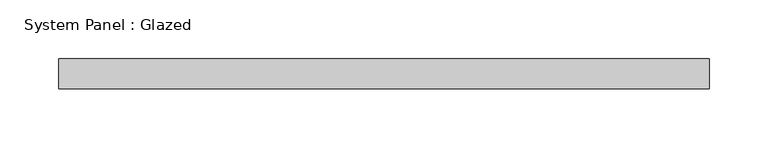
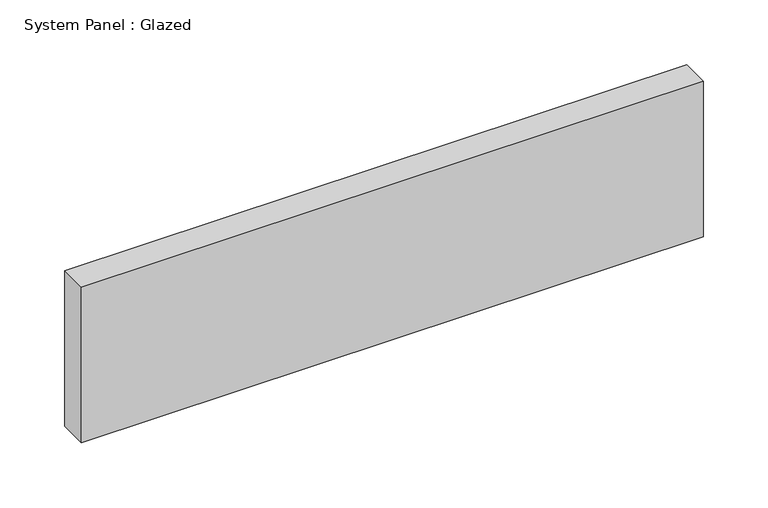
"""IFC4 building model written with IfcOpenShell, lengths in millimetres: plate geometry, System Panel : Glazed."""

from ifc_helpers import new_model, si_unit, origin, origin_with_axes, place, context, project, spatial, polyline, outline, extrude, source, transform, mapped, element, save


def system_panel_glazed_844a74e3(model_context):
    return source(origin(), model_context, "Body", "SweptSolid", [
        extrude(outline(polyline([(276.2250002, 19.05), (-276.2250002, 19.05), (-276.2250002, 44.45), (276.2250002, 44.45), (276.2250002, 19.05)])), origin_with_axes(), (0.0, 0.0, 1.0), 146.05),
    ])


if __name__ == "__main__":
    model = new_model("IFC4")
    model_context = context("Model", 3, world=origin())
    ifc_project = project(units=[si_unit("LENGTHUNIT", "METRE", prefix="MILLI")], contexts=[model_context])
    site = spatial("IfcSite", under=ifc_project)
    building = spatial("IfcBuilding", under=site)
    placement = place(None, origin())
    system_panel_glazed_shape = system_panel_glazed_844a74e3(model_context)
    element("IfcPlate", 1, ObjectType="System Panel : Glazed", at=placement, inside=building, context=model_context, shape_type="MappedRepresentation", body=[
        mapped(system_panel_glazed_shape, transform((0.0, 0.0, 0.0), x_axis=(1.0, 0.0, 0.0), y_axis=(0.0, 1.0, 0.0), z_axis=(0.0, 0.0, 1.0))),
    ])
    save(model, "model.ifc")

# Revit data of these elements
# Type "System Panel : Glazed"
#   Construction Type Id = "GSP4R"
#   Analytic Construction = "1/8 in Pilkington single glazing"
#   Visual Light Transmittance = 0.9
#   Solar Heat Gain Coefficient = 0.86
#   Heat Transfer Coefficient (U) = 1.18115 BTU/(h·ft²·°F)
#   Define Thermal Properties by = 1
# Element 1 (IfcPlate, "System Panel : Glazed")
#   Materials on its faces: "Glass"
# Materials
#   "Glass": class "Glass", colour RGB 0 128 192, transparency 0.75, Description = "Soda Lime Glass", Cost = 0
